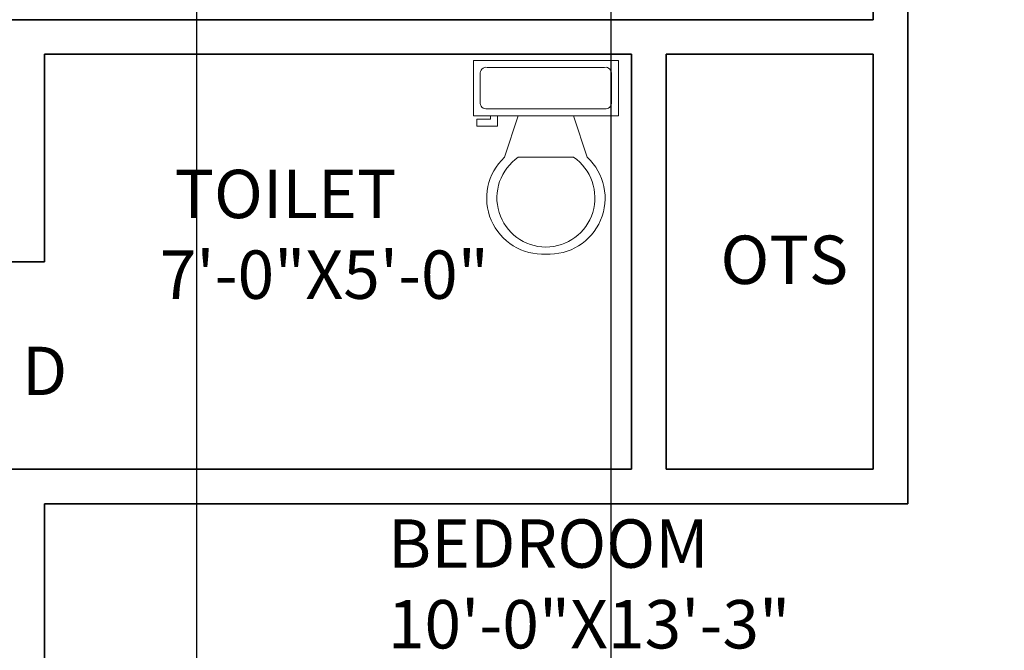
# Model space of a CAD drawing. Units: inches. Extents: x 3731 to 4318, y 1310 to 2388.
# Tile 14 of 57: x 3944 to 4086, y 1463 to 1554. Entities that reach past the tile are written whole.
import ezdxf

# ---------------------------------------------------------------- set-up
doc = ezdxf.new("R2010")
doc.units = ezdxf.units.IN
for name, color, linetype, lineweight in [('A-ANNO-DIMS', 2, 'Continuous', 18), ('A-ANNO-TEXT', 7, 'Continuous', 18), ('A-AREA-IDEN', 7, 'Continuous', 18), ('A-FLOR-FIXT', 9, 'Continuous', 18), ('A-WALL', 7, 'Continuous', 35)]:
    doc.layers.add(name, color=color, linetype=linetype, lineweight=lineweight)
doc.styles.get("Standard").update_dxf_attribs({"font": 'arial.ttf'})
doc.dimstyles.get("Standard").update_dxf_attribs({"dimtxt": 0.18, "dimasz": 0.18, "dimexe": 0.18, "dimexo": 0.0625, "dimgap": 0.09, "dimtad": 0, "dimtih": 1, "dimtoh": 1, "dimdec": 4, "dimzin": 0, "dimdsep": 46, "dimtxsty": 'Standard', "dimcen": 0.09, "dimadec": 0, "dimazin": 0, "dimtfac": 1, "dimtdec": 4, "dimtofl": 0, "dimtmove": 0, "dimatfit": 3, "dimfxl": 1, "dimtolj": 1, "dimtzin": 0, "dimarcsym": 0})

# ---------------------------------------------------------------- blocks, each defined once
blk = doc.blocks.new('*U14')
for p, q in [((9.5, -6), (9.5, -2)), ((-10, -8.5), (-8, -8.5)), ((-10, -9.5), (-10, -8.5)), ((-8, -8.5), (-8, -8)), ((-7, -8), (-7, -9.5)), ((-4, -8), (-6, -14)), ((4, -8), (6, -14)), ((-7, -9.5), (-10, -9.5)), ((4, -14), (-4, -14))]:
    blk.add_line(p, q)
blk.add_lwpolyline([(10.5, -8), (10.5, 0), (-10.5, 0), (-10.5, -8)], close=True)
for points in [[(8.5, -1), (-8.5, -1)], [(-9.5, -2), (-9.5, -6)], [(-8.5, -7), (8.5, -7)]]:
    blk.add_lwpolyline(points)
for centre, radius, start, end in [((-8.625, -1.875), 0.8839, 81.8699, 188.1301), ((8.625, -1.875), 0.8839, 351.8699, 98.1301), ((-8.625, -6.125), 0.8839, 171.869898, 278.1301), ((8.625, -6.125), 0.8839, 261.8699, 8.1301), ((-0.4772, -19.9188), 8.0953, 133.01722, 273.38), ((0.0374, -19.8731), 7.127, 124.50543, 269.7), ((-0.0373, -19.8731), 7.127, 270.3, 55.4946), ((0.4773, -19.9188), 8.0953, 266.62, 46.9828)]:
    blk.add_arc(centre, radius, start, end)
blk = doc.blocks.new('*D32')
at = {"layer": 'A-ANNO-DIMS', "color": 0, "lineweight": -2, "transparency": 16777216}
for p, q in [((4269.21, 1592.32), (4269.21, 1310.25)), ((3835.21, 1359.32), (3835.21, 1310.25)), ((3835.39, 1310.43), (4051.92, 1310.43)), ((4269.03, 1310.43), (4052.5, 1310.43))]:
    blk.add_line(p, q, dxfattribs=at)
at = {"layer": 'A-ANNO-DIMS', "color": 0, "transparency": 16777216}
for points in [[(3835.39, 1310.46), (3835.39, 1310.4), (3835.21, 1310.43)], [(4269.03, 1310.46), (4269.03, 1310.4), (4269.21, 1310.43)]]:
    blk.add_solid(points, dxfattribs=at)
at = {"layer": 'Defpoints', "color": 0, "transparency": 16777216}
for p in [(4269.21, 1592.38), (3835.21, 1359.38), (4269.21, 1310.43)]:
    blk.add_point(p, dxfattribs=at)
at = {"layer": 'A-ANNO-DIMS', "color": 0, "transparency": 16777216, "insert": (4052.21, 1310.43), "char_height": 0.18, "attachment_point": 5}
blk.add_mtext('\\A1;434', dxfattribs=at)
blk = doc.blocks.new('*D44')
at = {"layer": 'A-ANNO-DIMS', "color": 0, "lineweight": -2, "transparency": 16777216}
for p, q in [((3969.21, 1874.32), (3969.21, 1310.25)), ((4029.21, 1874.32), (4029.21, 1310.25)), ((3969.39, 1310.43), (3998.99, 1310.43)), ((4029.03, 1310.43), (3999.43, 1310.43))]:
    blk.add_line(p, q, dxfattribs=at)
at = {"layer": 'A-ANNO-DIMS', "color": 0, "transparency": 16777216}
for points in [[(3969.39, 1310.46), (3969.39, 1310.4), (3969.21, 1310.43)], [(4029.03, 1310.46), (4029.03, 1310.4), (4029.21, 1310.43)]]:
    blk.add_solid(points, dxfattribs=at)
at = {"layer": 'Defpoints', "color": 0, "transparency": 16777216}
for p in [(3969.21, 1874.38), (4029.21, 1874.38), (4029.21, 1310.43)]:
    blk.add_point(p, dxfattribs=at)
at = {"layer": 'A-ANNO-DIMS', "color": 0, "transparency": 16777216, "insert": (3999.21, 1310.43), "char_height": 0.18, "attachment_point": 5}
blk.add_mtext('\\A1;60', dxfattribs=at)

msp = doc.modelspace()

# ---------------------------------------------------------------- linework, layer by layer
at = {"layer": 'A-WALL'}
for p, q in [((4067.21, 1803.38), (4067.21, 1554.38)), ((4072.21, 1803.38), (4072.21, 1484.38)), ((3942.21, 1554.38), (4067.21, 1554.38)), ((3947.21, 1549.38), (3947.21, 1519.38)), ((3947.21, 1549.38), (4032.21, 1549.38)), ((4032.21, 1549.38), (4032.21, 1489.38)), ((4037.21, 1549.38), (4037.21, 1489.38)), ((4037.21, 1549.38), (4067.21, 1549.38)), ((4067.21, 1549.38), (4067.21, 1489.38)), ((3942.21, 1519.38), (3947.21, 1519.38)), ((3942.21, 1489.38), (4032.21, 1489.38)), ((4037.21, 1489.38), (4067.21, 1489.38)), ((3947.21, 1484.38), (4072.21, 1484.38)), ((3947.21, 1484.38), (3947.21, 1364.38))]:
    msp.add_line(p, q, dxfattribs=at)

# ---------------------------------------------------------------- block references
at = {"layer": 'A-FLOR-FIXT'}
msp.add_blockref('*U14', (4019.81, 1548.49), dxfattribs=at)

# ---------------------------------------------------------------- texts
at = {"layer": 'A-ANNO-TEXT', "insert": (3943.95, 1507.09), "char_height": 7, "attachment_point": 1}
msp.add_mtext_dynamic_manual_height_columns('D', width=10.4564, gutter_width=12.5, heights=[0], dxfattribs=at)
at = {"layer": 'A-AREA-IDEN', "char_height": 7, "attachment_point": 1}
for s, width, insert in [(' TOILET\\P7\'-0"X5\'-0"', 39.1687, (3963.9, 1532.68)), ('OTS', 47.0437, (4045.08, 1523.16)), ('BEDROOM\\P10\'-0"X13\'-3"', 47.0437, (3996.93, 1482.12))]:
    msp.add_mtext_dynamic_manual_height_columns(s, width=width, gutter_width=12.5, heights=[0], dxfattribs=dict(at, insert=insert))

# ---------------------------------------------------------------- dimensions: what is measured, and where the dimension line sits
at = {"layer": 'A-ANNO-DIMS'}
for base, p1, p2, picture, middle in [((4029.21, 1310.43), (3969.21, 1874.38), (4029.21, 1874.38), '*D44', (3999.21, 1310.43)), ((4269.21, 1310.43), (3835.21, 1359.38), (4269.21, 1592.38), '*D32', (4052.21, 1310.43))]:
    dim = msp.add_linear_dim(base=base, p1=p1, p2=p2, dimstyle='Standard', override={"dimdec": 0, "dimlfac": 1, "dimrnd": 0, "dimzin": 0, "dimdsep": 46, "dimlunit": 2}, dxfattribs=at)
    dim.commit()
    dim.dimension.update_dxf_attribs({"geometry": picture, "text_midpoint": middle})

doc.saveas('drawing.dxf')
